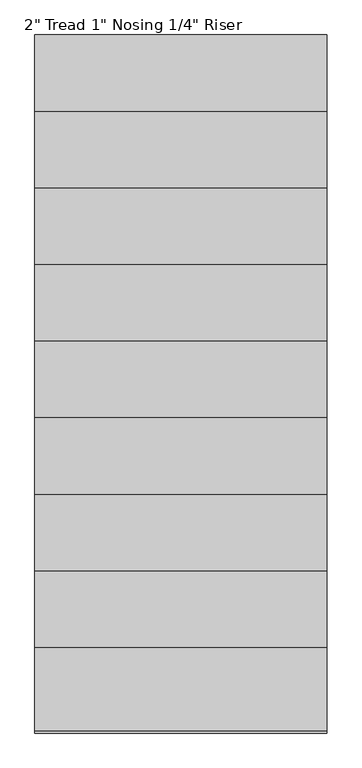
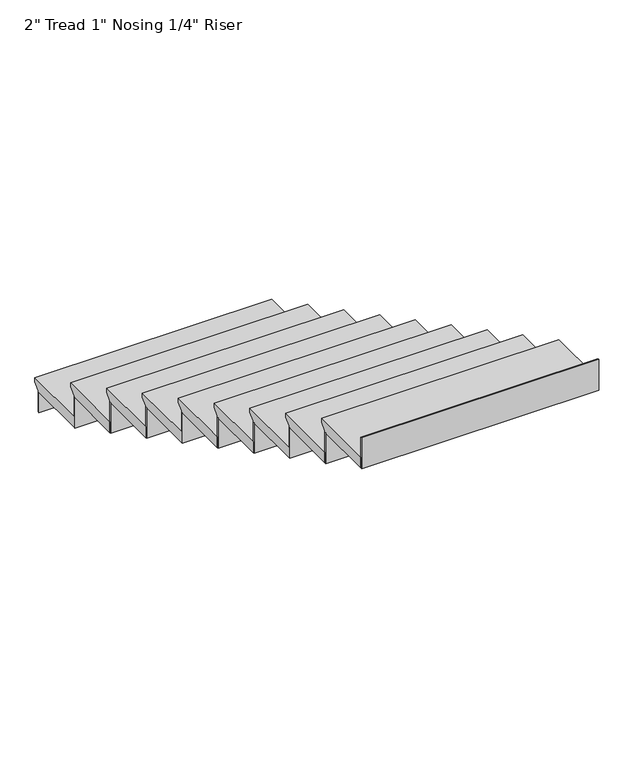
"""IFC4 building model written with IfcOpenShell, lengths in millimetres: stair flight geometry."""

from ifc_helpers import new_model, si_unit, origin, place, context, project, spatial, faceted_brep, source, transform, mapped, element, save


def stair_flight_4edc9e4a(model_context):
    return source(origin(), model_context, "Body", "Brep", [
        faceted_brep([(-16114.6847893, 12510.5922903, 3326.8227273), (-16114.6847893, 12510.5922903, 3345.8727273), (-15047.8847893, 12510.5922903, 3345.8727273), (-15047.8847893, 12510.5922903, 3326.8227273), (-16114.6847893, 12485.1922903, 3301.4227273), (-15047.8847893, 12485.1922903, 3301.4227273), (-16114.6847893, 12205.7922903, 3345.8727273), (-15047.8847893, 12205.7922903, 3345.8727273), (-15047.8847893, 12485.1922903, 3295.0727273), (-15047.8847893, 12205.7922903, 3295.0727273), (-16114.6847893, 12205.7922903, 3295.0727273), (-16114.6847893, 12485.1922903, 3295.0727273)], [[[0, 1, 2, 3]], [[4, 0, 3, 5]], [[2, 1, 6, 7]], [[8, 9, 10, 11]], [[2, 7, 9, 8, 5, 3]], [[8, 11, 4, 5]], [[6, 1, 0, 4, 11, 10]], [[7, 6, 10, 9]]]),
        faceted_brep([(-16114.6847893, 12485.1922903, 3295.0727273), (-16114.6847893, 12485.1922903, 3200.4), (-16114.6847893, 12478.8422903, 3200.4), (-16114.6847893, 12478.8422903, 3295.0727273), (-15047.8847893, 12485.1922903, 3295.0727273), (-15047.8847893, 12478.8422903, 3295.0727273), (-15047.8847893, 12478.8422903, 3200.4), (-15047.8847893, 12485.1922903, 3200.4)], [[[0, 1, 2, 3]], [[4, 5, 6, 7]], [[1, 0, 4, 7]], [[2, 1, 7, 6]], [[3, 2, 6, 5]], [[0, 3, 5, 4]]]),
        faceted_brep([(-16114.6847893, 12205.7922903, 3440.5454545), (-16114.6847893, 12205.7922903, 3295.0727273), (-16114.6847893, 12199.4422903, 3295.0727273), (-16114.6847893, 12199.4422903, 3440.5454545), (-15047.8847893, 12205.7922903, 3440.5454545), (-15047.8847893, 12199.4422903, 3440.5454545), (-15047.8847893, 12199.4422903, 3295.0727273), (-15047.8847893, 12205.7922903, 3295.0727273)], [[[0, 1, 2, 3]], [[4, 5, 6, 7]], [[1, 0, 4, 7]], [[2, 1, 7, 6]], [[3, 2, 6, 5]], [[0, 3, 5, 4]]]),
        faceted_brep([(-15047.8847893, 12231.1922903, 3491.3454545), (-16114.6847893, 12231.1922903, 3491.3454545), (-16114.6847893, 11926.3922903, 3491.3454545), (-15047.8847893, 11926.3922903, 3491.3454545), (-15047.8847893, 12205.7922903, 3440.5454545), (-15047.8847893, 11926.3922903, 3440.5454545), (-16114.6847893, 11926.3922903, 3440.5454545), (-16114.6847893, 12205.7922903, 3440.5454545), (-15047.8847893, 12205.7922903, 3446.8954545), (-15047.8847893, 12231.1922903, 3472.2954545), (-16114.6847893, 12205.7922903, 3446.8954545), (-16114.6847893, 12231.1922903, 3472.2954545)], [[[0, 1, 2, 3]], [[4, 5, 6, 7]], [[0, 3, 5, 4, 8, 9]], [[4, 7, 10, 8]], [[2, 1, 11, 10, 7, 6]], [[3, 2, 6, 5]], [[11, 1, 0, 9]], [[10, 11, 9, 8]]]),
        faceted_brep([(-16114.6847893, 11926.3922903, 3586.0181818), (-16114.6847893, 11926.3922903, 3440.5454545), (-16114.6847893, 11920.0422903, 3440.5454545), (-16114.6847893, 11920.0422903, 3586.0181818), (-15047.8847893, 11926.3922903, 3586.0181818), (-15047.8847893, 11920.0422903, 3586.0181818), (-15047.8847893, 11920.0422903, 3440.5454545), (-15047.8847893, 11926.3922903, 3440.5454545)], [[[0, 1, 2, 3]], [[4, 5, 6, 7]], [[1, 0, 4, 7]], [[2, 1, 7, 6]], [[3, 2, 6, 5]], [[0, 3, 5, 4]]]),
        faceted_brep([(-15047.8847893, 11951.7922903, 3636.8181818), (-16114.6847893, 11951.7922903, 3636.8181818), (-16114.6847893, 11646.9922903, 3636.8181818), (-15047.8847893, 11646.9922903, 3636.8181818), (-15047.8847893, 11926.3922903, 3586.0181818), (-15047.8847893, 11646.9922903, 3586.0181818), (-16114.6847893, 11646.9922903, 3586.0181818), (-16114.6847893, 11926.3922903, 3586.0181818), (-15047.8847893, 11926.3922903, 3592.3681818), (-15047.8847893, 11951.7922903, 3617.7681818), (-16114.6847893, 11926.3922903, 3592.3681818), (-16114.6847893, 11951.7922903, 3617.7681818)], [[[0, 1, 2, 3]], [[4, 5, 6, 7]], [[0, 3, 5, 4, 8, 9]], [[4, 7, 10, 8]], [[2, 1, 11, 10, 7, 6]], [[3, 2, 6, 5]], [[11, 1, 0, 9]], [[10, 11, 9, 8]]]),
        faceted_brep([(-16114.6847893, 11646.9922903, 3731.4909091), (-16114.6847893, 11646.9922903, 3586.0181818), (-16114.6847893, 11640.6422903, 3586.0181818), (-16114.6847893, 11640.6422903, 3731.4909091), (-15047.8847893, 11646.9922903, 3731.4909091), (-15047.8847893, 11640.6422903, 3731.4909091), (-15047.8847893, 11640.6422903, 3586.0181818), (-15047.8847893, 11646.9922903, 3586.0181818)], [[[0, 1, 2, 3]], [[4, 5, 6, 7]], [[1, 0, 4, 7]], [[2, 1, 7, 6]], [[3, 2, 6, 5]], [[0, 3, 5, 4]]]),
        faceted_brep([(-15047.8847893, 11672.3922903, 3782.2909091), (-16114.6847893, 11672.3922903, 3782.2909091), (-16114.6847893, 11367.5922903, 3782.2909091), (-15047.8847893, 11367.5922903, 3782.2909091), (-15047.8847893, 11646.9922903, 3731.4909091), (-15047.8847893, 11367.5922903, 3731.4909091), (-16114.6847893, 11367.5922903, 3731.4909091), (-16114.6847893, 11646.9922903, 3731.4909091), (-15047.8847893, 11646.9922903, 3737.8409091), (-15047.8847893, 11672.3922903, 3763.2409091), (-16114.6847893, 11646.9922903, 3737.8409091), (-16114.6847893, 11672.3922903, 3763.2409091)], [[[0, 1, 2, 3]], [[4, 5, 6, 7]], [[0, 3, 5, 4, 8, 9]], [[4, 7, 10, 8]], [[2, 1, 11, 10, 7, 6]], [[3, 2, 6, 5]], [[11, 1, 0, 9]], [[10, 11, 9, 8]]]),
        faceted_brep([(-16114.6847893, 11367.5922903, 3876.9636364), (-16114.6847893, 11367.5922903, 3731.4909091), (-16114.6847893, 11361.2422903, 3731.4909091), (-16114.6847893, 11361.2422903, 3876.9636364), (-15047.8847893, 11367.5922903, 3876.9636364), (-15047.8847893, 11361.2422903, 3876.9636364), (-15047.8847893, 11361.2422903, 3731.4909091), (-15047.8847893, 11367.5922903, 3731.4909091)], [[[0, 1, 2, 3]], [[4, 5, 6, 7]], [[1, 0, 4, 7]], [[2, 1, 7, 6]], [[3, 2, 6, 5]], [[0, 3, 5, 4]]]),
        faceted_brep([(-15047.8847893, 11392.9922903, 3927.7636364), (-16114.6847893, 11392.9922903, 3927.7636364), (-16114.6847893, 11088.1922903, 3927.7636364), (-15047.8847893, 11088.1922903, 3927.7636364), (-15047.8847893, 11367.5922903, 3876.9636364), (-15047.8847893, 11088.1922903, 3876.9636364), (-16114.6847893, 11088.1922903, 3876.9636364), (-16114.6847893, 11367.5922903, 3876.9636364), (-15047.8847893, 11367.5922903, 3883.3136364), (-15047.8847893, 11392.9922903, 3908.7136364), (-16114.6847893, 11367.5922903, 3883.3136364), (-16114.6847893, 11392.9922903, 3908.7136364)], [[[0, 1, 2, 3]], [[4, 5, 6, 7]], [[0, 3, 5, 4, 8, 9]], [[4, 7, 10, 8]], [[2, 1, 11, 10, 7, 6]], [[3, 2, 6, 5]], [[11, 1, 0, 9]], [[10, 11, 9, 8]]]),
        faceted_brep([(-16114.6847893, 11088.1922903, 4022.4363636), (-16114.6847893, 11088.1922903, 3876.9636364), (-16114.6847893, 11081.8422903, 3876.9636364), (-16114.6847893, 11081.8422903, 4022.4363636), (-15047.8847893, 11088.1922903, 4022.4363636), (-15047.8847893, 11081.8422903, 4022.4363636), (-15047.8847893, 11081.8422903, 3876.9636364), (-15047.8847893, 11088.1922903, 3876.9636364)], [[[0, 1, 2, 3]], [[4, 5, 6, 7]], [[1, 0, 4, 7]], [[2, 1, 7, 6]], [[3, 2, 6, 5]], [[0, 3, 5, 4]]]),
        faceted_brep([(-15047.8847893, 11113.5922903, 4073.2363636), (-16114.6847893, 11113.5922903, 4073.2363636), (-16114.6847893, 10808.7922903, 4073.2363636), (-15047.8847893, 10808.7922903, 4073.2363636), (-15047.8847893, 11088.1922903, 4022.4363636), (-15047.8847893, 10808.7922903, 4022.4363636), (-16114.6847893, 10808.7922903, 4022.4363636), (-16114.6847893, 11088.1922903, 4022.4363636), (-15047.8847893, 11088.1922903, 4028.7863636), (-15047.8847893, 11113.5922903, 4054.1863636), (-16114.6847893, 11088.1922903, 4028.7863636), (-16114.6847893, 11113.5922903, 4054.1863636)], [[[0, 1, 2, 3]], [[4, 5, 6, 7]], [[0, 3, 5, 4, 8, 9]], [[4, 7, 10, 8]], [[2, 1, 11, 10, 7, 6]], [[3, 2, 6, 5]], [[11, 1, 0, 9]], [[10, 11, 9, 8]]]),
        faceted_brep([(-16114.6847893, 10808.7922903, 4167.9090909), (-16114.6847893, 10808.7922903, 4022.4363636), (-16114.6847893, 10802.4422903, 4022.4363636), (-16114.6847893, 10802.4422903, 4167.9090909), (-15047.8847893, 10808.7922903, 4167.9090909), (-15047.8847893, 10802.4422903, 4167.9090909), (-15047.8847893, 10802.4422903, 4022.4363636), (-15047.8847893, 10808.7922903, 4022.4363636)], [[[0, 1, 2, 3]], [[4, 5, 6, 7]], [[1, 0, 4, 7]], [[2, 1, 7, 6]], [[3, 2, 6, 5]], [[0, 3, 5, 4]]]),
        faceted_brep([(-15047.8847893, 10834.1922903, 4218.7090909), (-16114.6847893, 10834.1922903, 4218.7090909), (-16114.6847893, 10529.3922903, 4218.7090909), (-15047.8847893, 10529.3922903, 4218.7090909), (-15047.8847893, 10808.7922903, 4167.9090909), (-15047.8847893, 10529.3922903, 4167.9090909), (-16114.6847893, 10529.3922903, 4167.9090909), (-16114.6847893, 10808.7922903, 4167.9090909), (-15047.8847893, 10808.7922903, 4174.2590909), (-15047.8847893, 10834.1922903, 4199.6590909), (-16114.6847893, 10808.7922903, 4174.2590909), (-16114.6847893, 10834.1922903, 4199.6590909)], [[[0, 1, 2, 3]], [[4, 5, 6, 7]], [[0, 3, 5, 4, 8, 9]], [[4, 7, 10, 8]], [[2, 1, 11, 10, 7, 6]], [[3, 2, 6, 5]], [[11, 1, 0, 9]], [[10, 11, 9, 8]]]),
        faceted_brep([(-16114.6847893, 10529.3922903, 4313.3818182), (-16114.6847893, 10529.3922903, 4167.9090909), (-16114.6847893, 10523.0422903, 4167.9090909), (-16114.6847893, 10523.0422903, 4313.3818182), (-15047.8847893, 10529.3922903, 4313.3818182), (-15047.8847893, 10523.0422903, 4313.3818182), (-15047.8847893, 10523.0422903, 4167.9090909), (-15047.8847893, 10529.3922903, 4167.9090909)], [[[0, 1, 2, 3]], [[4, 5, 6, 7]], [[1, 0, 4, 7]], [[2, 1, 7, 6]], [[3, 2, 6, 5]], [[0, 3, 5, 4]]]),
        faceted_brep([(-15047.8847893, 10554.7922903, 4364.1818182), (-16114.6847893, 10554.7922903, 4364.1818182), (-16114.6847893, 10249.9922903, 4364.1818182), (-15047.8847893, 10249.9922903, 4364.1818182), (-15047.8847893, 10529.3922903, 4313.3818182), (-15047.8847893, 10249.9922903, 4313.3818182), (-16114.6847893, 10249.9922903, 4313.3818182), (-16114.6847893, 10529.3922903, 4313.3818182), (-15047.8847893, 10529.3922903, 4319.7318182), (-15047.8847893, 10554.7922903, 4345.1318182), (-16114.6847893, 10529.3922903, 4319.7318182), (-16114.6847893, 10554.7922903, 4345.1318182)], [[[0, 1, 2, 3]], [[4, 5, 6, 7]], [[0, 3, 5, 4, 8, 9]], [[4, 7, 10, 8]], [[2, 1, 11, 10, 7, 6]], [[3, 2, 6, 5]], [[11, 1, 0, 9]], [[10, 11, 9, 8]]]),
        faceted_brep([(-16114.6847893, 9970.5922903, 4604.3272727), (-16114.6847893, 9970.5922903, 4458.8545455), (-16114.6847893, 9964.2422903, 4458.8545455), (-16114.6847893, 9964.2422903, 4604.3272727), (-15047.8847893, 9970.5922903, 4604.3272727), (-15047.8847893, 9964.2422903, 4604.3272727), (-15047.8847893, 9964.2422903, 4458.8545455), (-15047.8847893, 9970.5922903, 4458.8545455)], [[[0, 1, 2, 3]], [[4, 5, 6, 7]], [[1, 0, 4, 7]], [[2, 1, 7, 6]], [[3, 2, 6, 5]], [[0, 3, 5, 4]]]),
        faceted_brep([(-16114.6847893, 10249.9922903, 4458.8545455), (-16114.6847893, 10249.9922903, 4313.3818182), (-16114.6847893, 10243.6422903, 4313.3818182), (-16114.6847893, 10243.6422903, 4458.8545455), (-15047.8847893, 10249.9922903, 4458.8545455), (-15047.8847893, 10243.6422903, 4458.8545455), (-15047.8847893, 10243.6422903, 4313.3818182), (-15047.8847893, 10249.9922903, 4313.3818182)], [[[0, 1, 2, 3]], [[4, 5, 6, 7]], [[1, 0, 4, 7]], [[2, 1, 7, 6]], [[3, 2, 6, 5]], [[0, 3, 5, 4]]]),
        faceted_brep([(-15047.8847893, 9970.5922903, 4509.6545455), (-15047.8847893, 9995.9922903, 4509.6545455), (-15047.8847893, 10275.3922903, 4509.6545455), (-16114.6847893, 10275.3922903, 4509.6545455), (-16114.6847893, 9970.5922903, 4509.6545455), (-15047.8847893, 9995.9922903, 4458.8545455), (-15047.8847893, 9970.5922903, 4458.8545455), (-16114.6847893, 9970.5922903, 4458.8545455), (-16114.6847893, 10249.9922903, 4458.8545455), (-15047.8847893, 10249.9922903, 4458.8545455), (-15047.8847893, 10249.9922903, 4465.2045455), (-15047.8847893, 10275.3922903, 4490.6045455), (-16114.6847893, 10249.9922903, 4465.2045455), (-16114.6847893, 10275.3922903, 4490.6045455)], [[[0, 1, 2, 3, 4]], [[5, 6, 7, 8, 9]], [[1, 0, 6, 5]], [[2, 1, 5, 9, 10, 11]], [[9, 8, 12, 10]], [[4, 3, 13, 12, 8, 7]], [[0, 4, 7, 6]], [[13, 3, 2, 11]], [[12, 13, 11, 10]]]),
    ])


if __name__ == "__main__":
    model = new_model("IFC4")
    model_context = context("Model", 3, world=origin())
    ifc_project = project(units=[si_unit("LENGTHUNIT", "METRE", prefix="MILLI")], contexts=[model_context])
    site = spatial("IfcSite", under=ifc_project)
    building = spatial("IfcBuilding", under=site)
    placement = place(None, origin())
    stair_flight_shape = stair_flight_4edc9e4a(model_context)
    element("IfcStairFlight", 1, ObjectType="2\" Tread 1\" Nosing 1/4\" Riser", at=placement, inside=building, context=model_context, shape_type="MappedRepresentation", body=[
        mapped(stair_flight_shape, transform((0.0, 0.0, 0.0), x_axis=(1.0, 0.0, 0.0), y_axis=(0.0, 1.0, 0.0), z_axis=(0.0, 0.0, 1.0))),
    ])
    save(model, "model.ifc")
